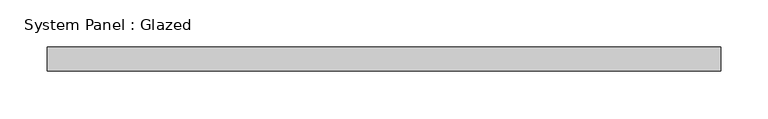
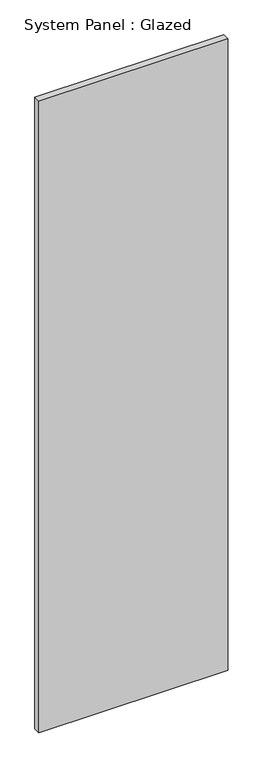
"""IFC4 building model written with IfcOpenShell, lengths in millimetres: plate geometry, System Panel : Glazed."""

from ifc_helpers import new_model, si_unit, origin, origin_with_axes, place, context, project, spatial, polyline, outline, extrude, source, transform, mapped, element, save


def system_panel_glazed_5a379f96(model_context):
    return source(origin(), model_context, "Body", "SweptSolid", [
        extrude(outline(polyline([(355.6000022, 19.05), (-355.6000022, 19.05), (-355.6000022, 44.45), (355.6000022, 44.45), (355.6000022, 19.05)])), origin_with_axes(), (0.0, 0.0, 1.0), 2514.6),
    ])


if __name__ == "__main__":
    model = new_model("IFC4")
    model_context = context("Model", 3, world=origin())
    ifc_project = project(units=[si_unit("LENGTHUNIT", "METRE", prefix="MILLI")], contexts=[model_context])
    site = spatial("IfcSite", under=ifc_project)
    building = spatial("IfcBuilding", under=site)
    placement = place(None, origin())
    system_panel_glazed_shape = system_panel_glazed_5a379f96(model_context)
    element("IfcPlate", 1, ObjectType="System Panel : Glazed", at=placement, inside=building, context=model_context, shape_type="MappedRepresentation", body=[
        mapped(system_panel_glazed_shape, transform((0.0, 0.0, 0.0), x_axis=(1.0, 0.0, 0.0), y_axis=(0.0, 1.0, 0.0), z_axis=(0.0, 0.0, 1.0))),
    ])
    save(model, "model.ifc")

# Revit data of these elements
# Type "System Panel : Glazed"
#   Construction Type Id = "GSP4R"
#   Analytic Construction = "1/8 in Pilkington single glazing"
#   Visual Light Transmittance = 0.9
#   Solar Heat Gain Coefficient = 0.86
#   Heat Transfer Coefficient (U) = 1.18115 BTU/(h·ft²·°F)
#   Define Thermal Properties by = 1
# Element 1 (IfcPlate, "System Panel : Glazed")
#   Materials on its faces: "Glass"
# Materials
#   "Glass": class "Glass", colour RGB 0 128 192, transparency 0.75, Description = "Soda Lime Glass", Cost = 0
